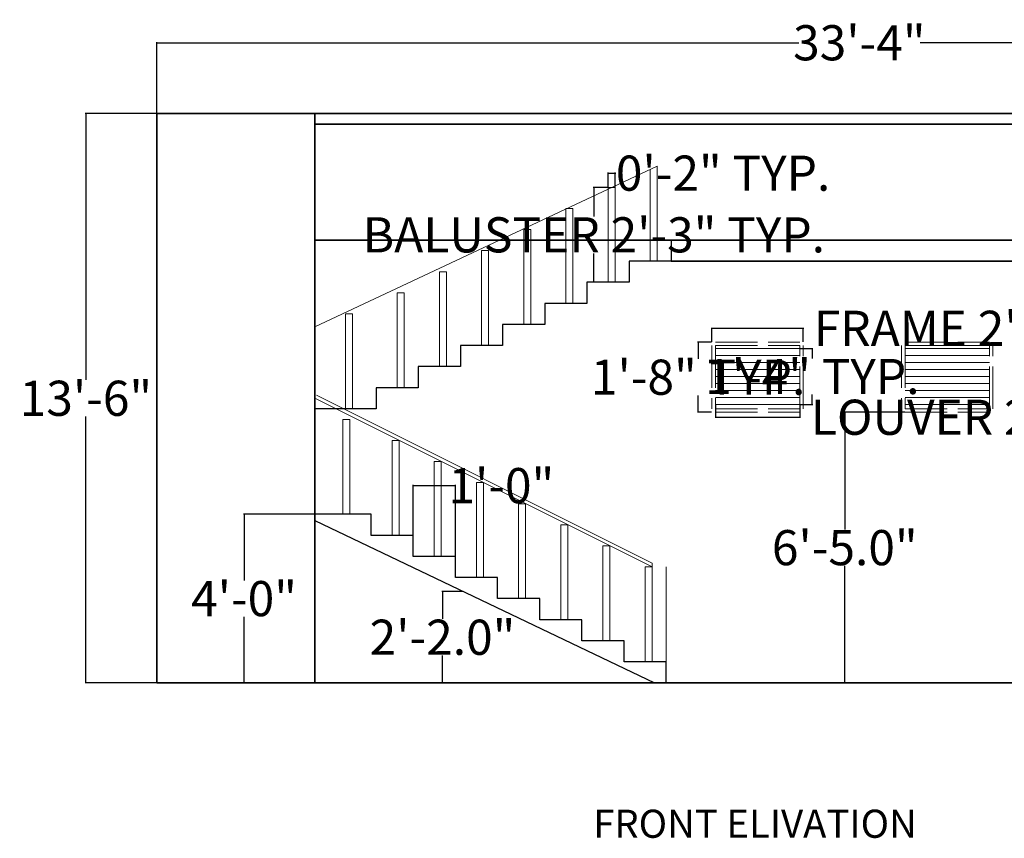
# Model space of a CAD drawing. Units: inches. Extents: x -413 to 212, y 1694 to 2633.
# Tile 1 of 5: x -378 to -98, y 1694 to 1927. Entities that reach past the tile are written whole.
import ezdxf

# ---------------------------------------------------------------- set-up
doc = ezdxf.new("R2010")
doc.units = ezdxf.units.IN
doc.header["$MEASUREMENT"] = 0
doc.linetypes.add('ACAD_ISO02W100', pattern=[15, 12, -3])
for name, color, linetype, lineweight in [('A-ANNO-DIMS', 5, 'Continuous', 18), ('A-ANNO-TEXT', 251, 'Continuous', 35), ('A-ELEV', 20, 'Continuous', 35), ('A-ELEV-RAIL', 3, 'Continuous', 18), ('A-ELEV-STRS', 3, 'Continuous', 25), ('A-ELEV-VENT', 2, 'Continuous', 18), ('A-ELEV-VENT-HIDN', 2, 'ACAD_ISO02W100', 18)]:
    doc.layers.add(name, color=color, linetype=linetype, lineweight=lineweight)
doc.styles.get("Standard").update_dxf_attribs({"font": 'arial.ttf'})
doc.dimstyles.get("Standard").update_dxf_attribs({"dimtxt": 10, "dimasz": 0.18, "dimexe": 0.18, "dimexo": 0.0625, "dimgap": 0.09, "dimtad": 0, "dimtih": 1, "dimtoh": 1, "dimdec": 1, "dimzin": 0, "dimdsep": 46, "dimlunit": 3, "dimtxsty": 'Standard', "dimblk": 'ARCHTICK', "dimcen": 0.09, "dimadec": 0, "dimazin": 0, "dimtfac": 1, "dimtdec": 1, "dimtofl": 0, "dimtmove": 0, "dimatfit": 3, "dimfxl": 1, "dimtolj": 1, "dimtzin": 0, "dimarcsym": 0})

# ---------------------------------------------------------------- blocks, each defined once
blk = doc.blocks.new('_ArchTick')
at = {"color": 0, "linetype": 'ByBlock', "const_width": 0.15}
blk.add_lwpolyline([(-0.5, -0.5), (0.5, 0.5)], dxfattribs=at)
blk = doc.blocks.new('*D9')
at = {"layer": 'A-ANNO-DIMS', "color": 0, "lineweight": -2, "transparency": 16777216}
for p, q in [((-126.04, 1815.59), (-143.33, 1815.59)), ((-143.15, 1815.59), (-143.15, 1782.28)), ((-143.15, 1738.59), (-143.15, 1771.89)), ((-126.04, 1738.59), (-143.33, 1738.59))]:
    blk.add_line(p, q, dxfattribs=at)
at = {"layer": 'Defpoints', "color": 0, "transparency": 16777216}
for p in [(-125.98, 1815.59), (-143.15, 1738.59), (-125.98, 1738.59)]:
    blk.add_point(p, dxfattribs=at)
at = {"layer": 'A-ANNO-DIMS', "color": 0, "lineweight": -2, "transparency": 16777216, "xscale": 0.18, "yscale": 0.18, "zscale": 0.18}
for p, rotation in [((-143.15, 1815.59), 90), ((-143.15, 1738.59), 270)]:
    blk.add_blockref('_ArchTick', p, dxfattribs=dict(at, rotation=rotation))
at = {"layer": 'A-ANNO-DIMS', "color": 0, "transparency": 16777216, "insert": (-143.15, 1777.09), "char_height": 10, "attachment_point": 5}
blk.add_mtext('\\A1;6\'-5.0"', dxfattribs=at)
blk = doc.blocks.new('*D10')
at = {"layer": 'A-ANNO-DIMS', "color": 0, "lineweight": -2, "transparency": 16777216}
for p, q in [((-251.8, 1764.61), (-257.82, 1764.61)), ((-257.64, 1764.61), (-257.64, 1756.79)), ((-257.64, 1738.59), (-257.64, 1746.4)), ((-252.43, 1738.59), (-257.82, 1738.59))]:
    blk.add_line(p, q, dxfattribs=at)
at = {"layer": 'Defpoints', "color": 0, "transparency": 16777216}
for p in [(-257.64, 1764.61), (-251.74, 1764.61), (-252.36, 1738.59)]:
    blk.add_point(p, dxfattribs=at)
at = {"layer": 'A-ANNO-DIMS', "color": 0, "lineweight": -2, "transparency": 16777216, "xscale": 0.18, "yscale": 0.18, "zscale": 0.18}
for p, rotation in [((-257.64, 1764.61), 90), ((-257.64, 1738.59), 270)]:
    blk.add_blockref('_ArchTick', p, dxfattribs=dict(at, rotation=rotation))
at = {"layer": 'A-ANNO-DIMS', "color": 0, "transparency": 16777216, "insert": (-257.64, 1751.6), "char_height": 10, "attachment_point": 5}
blk.add_mtext('\\A1;2\'-2.0"', dxfattribs=at)
blk = doc.blocks.new('VENT-FRAME-24X18-ELEV')
for p, q in [((1, 20), (25, 20)), ((0, 19), (0, 1)), ((1, 19), (25, 19)), ((1, 19), (1, 1)), ((25, 1), (25, 19)), ((26, 1), (26, 19)), ((1, 1), (25, 1)), ((1, 0), (25, 0))]:
    blk.add_line(p, q)
blk = doc.blocks.new('LOUVER-BLADES-24X18-ELEV')
for p, q in [((0, 16), (24, 16)), ((0, 14), (24, 14)), ((0, 12), (24, 12)), ((0, 10), (24, 10)), ((0, 8), (24, 8)), ((0, 6), (24, 6)), ((0, 4), (24, 4)), ((0, 2), (24, 2)), ((0, 0), (24, 0))]:
    blk.add_line(p, q)
blk = doc.blocks.new('BALUSTER-27IN-ELEV')
for p, q in [((0, 0), (0, 27)), ((0, 27), (2, 27)), ((2, 0), (2, 27))]:
    blk.add_line(p, q)
blk = doc.blocks.new('*D51')
at = {"layer": 'A-ANNO-DIMS', "color": 0, "lineweight": -2, "transparency": 16777216}
for p, q in [((-210.59, 1879.59), (-214.75, 1879.59)), ((-214.57, 1879.59), (-214.57, 1871.35)), ((-214.57, 1852.59), (-214.57, 1860.82)), ((-210.59, 1852.59), (-214.75, 1852.59))]:
    blk.add_line(p, q, dxfattribs=at)
at = {"layer": 'Defpoints', "color": 0, "transparency": 16777216}
for p in [(-214.57, 1879.59), (-210.52, 1879.59), (-210.52, 1852.59)]:
    blk.add_point(p, dxfattribs=at)
at = {"layer": 'A-ANNO-DIMS', "color": 0, "lineweight": -2, "transparency": 16777216, "xscale": 0.18, "yscale": 0.18, "zscale": 0.18}
for p, rotation in [((-214.57, 1879.59), 90), ((-214.57, 1852.59), 270)]:
    blk.add_blockref('_ArchTick', p, dxfattribs=dict(at, rotation=rotation))
at = {"layer": 'A-ANNO-DIMS', "color": 0, "transparency": 16777216, "insert": (-214.57, 1866.09), "char_height": 10, "attachment_point": 5}
blk.add_mtext('\\A1;BALUSTER 2\'-3" TYP.', dxfattribs=at)
blk = doc.blocks.new('*D52')
at = {"layer": 'A-ANNO-DIMS', "color": 0, "lineweight": -2, "transparency": 16777216}
for p, q in [((-210.52, 1879.65), (-210.52, 1883.82)), ((-210.52, 1883.64), (-208.52, 1883.64)), ((-208.52, 1879.65), (-208.52, 1883.82)), ((-208.52, 1883.64), (-208.34, 1883.64))]:
    blk.add_line(p, q, dxfattribs=at)
at = {"layer": 'Defpoints', "color": 0, "transparency": 16777216}
for p in [(-208.52, 1883.64), (-210.52, 1879.59), (-208.52, 1879.59)]:
    blk.add_point(p, dxfattribs=at)
at = {"layer": 'A-ANNO-DIMS', "color": 0, "lineweight": -2, "transparency": 16777216, "xscale": 0.18, "yscale": 0.18, "zscale": 0.18, "rotation": 180}
blk.add_blockref('_ArchTick', (-210.52, 1883.64), dxfattribs=at)
at = {"layer": 'A-ANNO-DIMS', "color": 0, "lineweight": -2, "transparency": 16777216, "xscale": 0.18, "yscale": 0.18, "zscale": 0.18}
blk.add_blockref('_ArchTick', (-208.52, 1883.64), dxfattribs=at)
at = {"layer": 'A-ANNO-DIMS', "color": 0, "transparency": 16777216, "insert": (-177.78, 1883.64), "char_height": 10, "attachment_point": 5}
blk.add_mtext('\\A1;0\'-2" TYP.', dxfattribs=at)
blk = doc.blocks.new('*D53')
at = {"layer": 'A-ANNO-DIMS', "color": 0, "lineweight": -2, "transparency": 16777216}
for p, q in [((-180.98, 1835.65), (-180.98, 1839.67)), ((-180.98, 1839.49), (-154.98, 1839.49)), ((-154.98, 1835.65), (-154.98, 1839.67)), ((-154.98, 1839.49), (-154.8, 1839.49))]:
    blk.add_line(p, q, dxfattribs=at)
at = {"layer": 'Defpoints', "color": 0, "transparency": 16777216}
for p in [(-154.98, 1839.49), (-180.98, 1835.59), (-154.98, 1835.59)]:
    blk.add_point(p, dxfattribs=at)
at = {"layer": 'A-ANNO-DIMS', "color": 0, "lineweight": -2, "transparency": 16777216, "xscale": 0.18, "yscale": 0.18, "zscale": 0.18, "rotation": 180}
blk.add_blockref('_ArchTick', (-180.98, 1839.49), dxfattribs=at)
at = {"layer": 'A-ANNO-DIMS', "color": 0, "lineweight": -2, "transparency": 16777216, "xscale": 0.18, "yscale": 0.18, "zscale": 0.18}
blk.add_blockref('_ArchTick', (-154.98, 1839.49), dxfattribs=at)
at = {"layer": 'A-ANNO-DIMS', "color": 0, "transparency": 16777216, "insert": (-98.12, 1839.49), "char_height": 10, "attachment_point": 5}
blk.add_mtext('\\A1;FRAME 2\'-2" TYP.', dxfattribs=at)
blk = doc.blocks.new('*D54')
at = {"layer": 'A-ANNO-DIMS', "color": 0, "lineweight": -2, "transparency": 16777216}
for p, q in [((-181.04, 1835.59), (-185.06, 1835.59)), ((-184.88, 1835.59), (-184.88, 1830.78)), ((-184.88, 1815.59), (-184.88, 1820.39)), ((-181.04, 1815.59), (-185.06, 1815.59))]:
    blk.add_line(p, q, dxfattribs=at)
at = {"layer": 'Defpoints', "color": 0, "transparency": 16777216}
for p in [(-184.88, 1835.59), (-180.98, 1835.59), (-180.98, 1815.59)]:
    blk.add_point(p, dxfattribs=at)
at = {"layer": 'A-ANNO-DIMS', "color": 0, "lineweight": -2, "transparency": 16777216, "xscale": 0.18, "yscale": 0.18, "zscale": 0.18}
for p, rotation in [((-184.88, 1835.59), 90), ((-184.88, 1815.59), 270)]:
    blk.add_blockref('_ArchTick', p, dxfattribs=dict(at, rotation=rotation))
at = {"layer": 'A-ANNO-DIMS', "color": 0, "transparency": 16777216, "insert": (-184.88, 1825.59), "char_height": 10, "attachment_point": 5}
blk.add_mtext('\\A1;1\'-8" TYP.', dxfattribs=at)
blk = doc.blocks.new('*D55')
at = {"layer": 'A-ANNO-DIMS', "color": 0, "lineweight": -2, "transparency": 16777216}
for p, q in [((-179.98, 1817.73), (-179.98, 1814.01)), ((-155.98, 1817.73), (-155.98, 1814.01)), ((-179.98, 1814.19), (-155.98, 1814.19)), ((-155.98, 1814.19), (-155.8, 1814.19))]:
    blk.add_line(p, q, dxfattribs=at)
at = {"layer": 'Defpoints', "color": 0, "transparency": 16777216}
for p in [(-179.98, 1817.79), (-155.98, 1817.79), (-155.98, 1814.19)]:
    blk.add_point(p, dxfattribs=at)
at = {"layer": 'A-ANNO-DIMS', "color": 0, "lineweight": -2, "transparency": 16777216, "xscale": 0.18, "yscale": 0.18, "zscale": 0.18, "rotation": 180}
blk.add_blockref('_ArchTick', (-179.98, 1814.19), dxfattribs=at)
at = {"layer": 'A-ANNO-DIMS', "color": 0, "lineweight": -2, "transparency": 16777216, "xscale": 0.18, "yscale": 0.18, "zscale": 0.18}
blk.add_blockref('_ArchTick', (-155.98, 1814.19), dxfattribs=at)
at = {"layer": 'A-ANNO-DIMS', "color": 0, "transparency": 16777216, "insert": (-94.78, 1814.19), "char_height": 10, "attachment_point": 5}
blk.add_mtext('\\A1;LOUVER 2\'-0" TYP.', dxfattribs=at)
blk = doc.blocks.new('*D56')
at = {"layer": 'A-ANNO-DIMS', "color": 0, "lineweight": -2, "transparency": 16777216}
for p, q in [((-155.91, 1833.79), (-152.2, 1833.79)), ((-152.38, 1833.79), (-152.38, 1830.9)), ((-152.38, 1817.79), (-152.38, 1820.68)), ((-155.91, 1817.79), (-152.2, 1817.79))]:
    blk.add_line(p, q, dxfattribs=at)
at = {"layer": 'Defpoints', "color": 0, "transparency": 16777216}
for p in [(-155.98, 1833.79), (-152.38, 1833.79), (-155.98, 1817.79)]:
    blk.add_point(p, dxfattribs=at)
at = {"layer": 'A-ANNO-DIMS', "color": 0, "lineweight": -2, "transparency": 16777216, "xscale": 0.18, "yscale": 0.18, "zscale": 0.18}
for p, rotation in [((-152.38, 1833.79), 90), ((-152.38, 1817.79), 270)]:
    blk.add_blockref('_ArchTick', p, dxfattribs=dict(at, rotation=rotation))
at = {"layer": 'A-ANNO-DIMS', "color": 0, "transparency": 16777216, "insert": (-152.38, 1825.79), "char_height": 10, "attachment_point": 5}
blk.add_mtext('\\A1;1\'-4" TYP.', dxfattribs=at)
blk = doc.blocks.new('*D60')
at = {"layer": 'A-ANNO-DIMS', "color": 0, "lineweight": -2, "transparency": 16777216}
for p, q in [((-338.98, 1900.65), (-338.98, 1920.92)), ((-338.98, 1920.74), (-156.26, 1920.74)), ((60.99, 1920.74), (-121.73, 1920.74)), ((60.99, 1900.65), (60.99, 1920.92))]:
    blk.add_line(p, q, dxfattribs=at)
at = {"layer": 'Defpoints', "color": 0, "transparency": 16777216}
for p in [(60.99, 1920.74), (-338.98, 1900.59), (60.99, 1900.59)]:
    blk.add_point(p, dxfattribs=at)
at = {"layer": 'A-ANNO-DIMS', "color": 0, "lineweight": -2, "transparency": 16777216, "xscale": 0.18, "yscale": 0.18, "zscale": 0.18, "rotation": 180}
blk.add_blockref('_ArchTick', (-338.98, 1920.74), dxfattribs=at)
at = {"layer": 'A-ANNO-DIMS', "color": 0, "lineweight": -2, "transparency": 16777216, "xscale": 0.18, "yscale": 0.18, "zscale": 0.18}
blk.add_blockref('_ArchTick', (60.99, 1920.74), dxfattribs=at)
at = {"layer": 'A-ANNO-DIMS', "color": 0, "transparency": 16777216, "insert": (-139, 1920.74), "char_height": 10, "attachment_point": 5}
blk.add_mtext('\\A1;33\'-4"', dxfattribs=at)
blk = doc.blocks.new('*D61')
at = {"layer": 'A-ANNO-DIMS', "color": 0, "lineweight": -2, "transparency": 16777216}
for p, q in [((-339.04, 1900.59), (-359.31, 1900.59)), ((-359.13, 1900.59), (-359.13, 1824.79)), ((-359.13, 1738.59), (-359.13, 1814.39)), ((-339.04, 1738.59), (-359.31, 1738.59))]:
    blk.add_line(p, q, dxfattribs=at)
at = {"layer": 'Defpoints', "color": 0, "transparency": 16777216}
for p in [(-359.13, 1900.59), (-338.98, 1900.59), (-338.98, 1738.59)]:
    blk.add_point(p, dxfattribs=at)
at = {"layer": 'A-ANNO-DIMS', "color": 0, "lineweight": -2, "transparency": 16777216, "xscale": 0.18, "yscale": 0.18, "zscale": 0.18}
for p, rotation in [((-359.13, 1900.59), 90), ((-359.13, 1738.59), 270)]:
    blk.add_blockref('_ArchTick', p, dxfattribs=dict(at, rotation=rotation))
at = {"layer": 'A-ANNO-DIMS', "color": 0, "transparency": 16777216, "insert": (-359.13, 1819.59), "char_height": 10, "attachment_point": 5}
blk.add_mtext('\\A1;13\'-6"', dxfattribs=at)
blk = doc.blocks.new('*D63')
at = {"layer": 'A-ANNO-DIMS', "color": 0, "lineweight": -2, "transparency": 16777216}
for p, q in [((-294.04, 1786.59), (-314.31, 1786.59)), ((-314.13, 1786.59), (-314.13, 1767.78)), ((-314.13, 1738.59), (-314.13, 1757.39)), ((-294.04, 1738.59), (-314.31, 1738.59))]:
    blk.add_line(p, q, dxfattribs=at)
at = {"layer": 'Defpoints', "color": 0, "transparency": 16777216}
for p in [(-314.13, 1786.59), (-293.98, 1786.59), (-293.98, 1738.59)]:
    blk.add_point(p, dxfattribs=at)
at = {"layer": 'A-ANNO-DIMS', "color": 0, "lineweight": -2, "transparency": 16777216, "xscale": 0.18, "yscale": 0.18, "zscale": 0.18}
for p, rotation in [((-314.13, 1786.59), 90), ((-314.13, 1738.59), 270)]:
    blk.add_blockref('_ArchTick', p, dxfattribs=dict(at, rotation=rotation))
at = {"layer": 'A-ANNO-DIMS', "color": 0, "transparency": 16777216, "insert": (-314.13, 1762.59), "char_height": 10, "attachment_point": 5}
blk.add_mtext('\\A1;4\'-0"', dxfattribs=at)
blk = doc.blocks.new('*D81')
at = {"layer": 'A-ANNO-DIMS', "color": 0, "lineweight": -2, "transparency": 16777216}
for p, q in [((-265.98, 1774.65), (-265.98, 1794.92)), ((-265.98, 1794.74), (-253.98, 1794.74)), ((-253.98, 1774.65), (-253.98, 1794.92)), ((-253.98, 1794.74), (-253.8, 1794.74))]:
    blk.add_line(p, q, dxfattribs=at)
at = {"layer": 'Defpoints', "color": 0, "transparency": 16777216}
for p in [(-253.98, 1794.74), (-265.98, 1774.59), (-253.98, 1774.59)]:
    blk.add_point(p, dxfattribs=at)
at = {"layer": 'A-ANNO-DIMS', "color": 0, "lineweight": -2, "transparency": 16777216, "xscale": 0.18, "yscale": 0.18, "zscale": 0.18, "rotation": 180}
blk.add_blockref('_ArchTick', (-265.98, 1794.74), dxfattribs=at)
at = {"layer": 'A-ANNO-DIMS', "color": 0, "lineweight": -2, "transparency": 16777216, "xscale": 0.18, "yscale": 0.18, "zscale": 0.18}
blk.add_blockref('_ArchTick', (-253.98, 1794.74), dxfattribs=at)
at = {"layer": 'A-ANNO-DIMS', "color": 0, "transparency": 16777216, "insert": (-240.89, 1794.74), "char_height": 10, "attachment_point": 5}
blk.add_mtext('\\A1;1\'-0"', dxfattribs=at)

msp = doc.modelspace()

# ---------------------------------------------------------------- linework, layer by layer
at = {"layer": 'A-ELEV'}
for p, q in [((-338.98, 1900.59), (60.99, 1900.59)), ((-338.98, 1900.59), (-338.98, 1738.59)), ((-293.98, 1900.59), (-293.98, 1738.59)), ((-293.98, 1897.59), (60.99, 1897.59)), ((-293.98, 1864.59), (60.99, 1864.59)), ((-192.52, 1858.59), (60.99, 1858.59)), ((-338.98, 1738.59), (60.99, 1738.59))]:
    msp.add_line(p, q, dxfattribs=at)
at = {"layer": 'A-ELEV-RAIL'}
for p, q in [((-196.52, 1885.59), (-293.98, 1839.92)), ((-198.52, 1858.59), (-198.52, 1884.65)), ((-196.52, 1858.59), (-196.52, 1885.59)), ((-197.98, 1771.59), (-293.98, 1819.59)), ((-197.98, 1772.71), (-293.53, 1820.48)), ((-199.98, 1744.59), (-199.98, 1771.59)), ((-199.98, 1771.59), (-197.98, 1771.59)), ((-197.98, 1744.59), (-197.98, 1772.71)), ((-193.98, 1744.59), (-193.98, 1771.59)), ((-193.98, 1771.59), (-193.98, 1738.59))]:
    msp.add_line(p, q, dxfattribs=at)
at = {"layer": 'A-ELEV-STRS'}
for p, q in [((-192.52, 1864.59), (-192.52, 1858.59)), ((-192.52, 1858.59), (-204.52, 1858.59)), ((-204.52, 1858.59), (-204.52, 1852.59)), ((-204.52, 1852.59), (-216.52, 1852.59)), ((-216.52, 1852.59), (-216.52, 1846.59)), ((-216.52, 1846.59), (-228.52, 1846.59)), ((-228.52, 1846.59), (-228.52, 1840.59)), ((-228.52, 1840.59), (-240.52, 1840.59)), ((-240.52, 1840.59), (-240.52, 1834.59)), ((-240.52, 1834.59), (-252.52, 1834.59)), ((-252.52, 1834.59), (-252.52, 1828.59)), ((-252.52, 1828.59), (-264.52, 1828.59)), ((-264.52, 1828.59), (-264.52, 1822.59)), ((-264.52, 1822.59), (-276.52, 1822.59)), ((-276.52, 1822.59), (-276.52, 1816.59)), ((-276.52, 1816.59), (-293.98, 1816.59)), ((-293.98, 1786.59), (-293.98, 1792.59)), ((-277.98, 1786.59), (-293.98, 1786.59)), ((-277.98, 1780.59), (-277.98, 1786.59)), ((-293.98, 1784.81), (-197.34, 1738.59)), ((-265.98, 1780.59), (-277.98, 1780.59)), ((-265.98, 1774.59), (-265.98, 1780.59)), ((-253.98, 1774.59), (-265.98, 1774.59)), ((-253.98, 1768.59), (-253.98, 1774.59)), ((-241.98, 1768.59), (-253.98, 1768.59)), ((-241.98, 1762.59), (-241.98, 1768.59)), ((-229.98, 1762.59), (-241.98, 1762.59)), ((-229.98, 1756.59), (-229.98, 1762.59)), ((-217.98, 1756.59), (-229.98, 1756.59)), ((-217.98, 1750.59), (-217.98, 1756.59)), ((-205.98, 1750.59), (-217.98, 1750.59)), ((-205.98, 1744.59), (-205.98, 1750.59)), ((-193.98, 1744.59), (-205.98, 1744.59)), ((-193.98, 1738.59), (-193.98, 1744.59))]:
    msp.add_line(p, q, dxfattribs=at)
at = {"layer": 'A-ELEV-VENT'}
msp.add_line((-155.98, 1833.79), (-154.98, 1833.79), dxfattribs=at)

# ---------------------------------------------------------------- block references
at = {"layer": 'A-ELEV-RAIL'}
for p in [(-210.52, 1852.59), (-222.52, 1846.59), (-234.52, 1840.59), (-246.52, 1834.59), (-258.52, 1828.59), (-270.52, 1822.59), (-285.25, 1816.59), (-285.98, 1786.59), (-271.98, 1780.59), (-259.98, 1774.59), (-247.98, 1768.59), (-235.98, 1762.59), (-223.98, 1756.59), (-211.98, 1750.59)]:
    msp.add_blockref('BALUSTER-27IN-ELEV', p, dxfattribs=at)
at = {"layer": 'A-ELEV-VENT'}
msp.add_blockref('LOUVER-BLADES-24X18-ELEV', (-179.98, 1817.79), dxfattribs=at)
at = {"layer": 'A-ELEV-VENT', "rotation": 180}
msp.add_blockref('LOUVER-BLADES-24X18-ELEV', (-101.98, 1833.79), dxfattribs=at)
at = {"layer": 'A-ELEV-VENT-HIDN'}
for p in [(-180.98, 1815.59), (-126.98, 1815.59)]:
    msp.add_blockref('VENT-FRAME-24X18-ELEV', p, dxfattribs=at)

# ---------------------------------------------------------------- texts
at = {"layer": 'A-ANNO-TEXT'}
msp.add_text('FRONT ELIVATION', height=8, dxfattribs=at).set_placement((-214.76, 1694.53))

# ---------------------------------------------------------------- dimensions: what is measured, and where the dimension line sits
at = {"layer": 'A-ANNO-DIMS'}
for base, p1, p2, picture, middle in [((60.99, 1920.74), (-338.98, 1900.59), (60.99, 1900.59), '*D60', (-139, 1920.74)), ((-253.98, 1794.74), (-265.98, 1774.59), (-253.98, 1774.59), '*D81', (-240.89, 1794.74))]:
    dim = msp.add_linear_dim(base=base, p1=p1, p2=p2, dimstyle='Standard', override={"dimdec": 1, "dimlfac": 1, "dimrnd": 0, "dimzin": 1, "dimdsep": 46, "dimlunit": 4, "dimfrac": 2}, dxfattribs=at)
    dim.commit()
    dim.dimension.update_dxf_attribs({"geometry": picture, "text_midpoint": middle})
for base, p1, p2, override, picture, middle in [((-359.13, 1900.59), (-338.98, 1738.59), (-338.98, 1900.59), {"dimdec": 1, "dimlfac": 1, "dimrnd": 0, "dimzin": 1, "dimdsep": 46, "dimlunit": 4, "dimfrac": 2}, '*D61', (-359.13, 1819.59)), ((-143.15, 1738.59), (-125.98, 1815.59), (-125.98, 1738.59), {"dimclrd": 0, "dimclre": 0, "dimclrt": 0}, '*D9', (-143.15, 1777.09)), ((-314.13, 1786.59), (-293.98, 1738.59), (-293.98, 1786.59), {"dimdec": 1, "dimlfac": 1, "dimrnd": 0, "dimzin": 1, "dimdsep": 46, "dimlunit": 4, "dimfrac": 2}, '*D63', (-314.13, 1762.59)), ((-257.64, 1764.61), (-252.36, 1738.59), (-251.74, 1764.61), {"dimclrd": 0, "dimclre": 0, "dimclrt": 0}, '*D10', (-257.64, 1751.6))]:
    dim = msp.add_linear_dim(base=base, p1=p1, p2=p2, angle=90, dimstyle='Standard', override=override, dxfattribs=at)
    dim.commit()
    dim.dimension.update_dxf_attribs({"geometry": picture, "text_midpoint": middle})
for base, p1, p2, text, picture, middle in [((-208.52, 1883.64), (-210.52, 1879.59), (-208.52, 1879.59), '<> TYP.', '*D52', (-177.78, 1883.64)), ((-154.98, 1839.49), (-180.98, 1835.59), (-154.98, 1835.59), 'FRAME <> TYP.', '*D53', (-98.12, 1839.49)), ((-155.98, 1814.19), (-179.98, 1817.79), (-155.98, 1817.79), 'LOUVER <> TYP.', '*D55', (-94.78, 1814.19))]:
    dim = msp.add_linear_dim(base=base, p1=p1, p2=p2, text=text, dimstyle='Standard', override={"dimdec": 1, "dimlfac": 1, "dimrnd": 0, "dimzin": 1, "dimdsep": 46, "dimlunit": 4, "dimfrac": 2}, dxfattribs=at)
    dim.commit()
    dim.dimension.update_dxf_attribs({"geometry": picture, "text_midpoint": middle})
for base, p1, p2, text, picture, middle in [((-214.57, 1879.59), (-210.52, 1852.59), (-210.52, 1879.59), 'BALUSTER <> TYP.', '*D51', (-214.57, 1866.09)), ((-184.88, 1835.59), (-180.98, 1815.59), (-180.98, 1835.59), '<> TYP.', '*D54', (-184.88, 1825.59)), ((-152.38, 1833.79), (-155.98, 1817.79), (-155.98, 1833.79), '<> TYP.', '*D56', (-152.38, 1825.79))]:
    dim = msp.add_linear_dim(base=base, p1=p1, p2=p2, angle=90, text=text, dimstyle='Standard', override={"dimdec": 1, "dimlfac": 1, "dimrnd": 0, "dimzin": 1, "dimdsep": 46, "dimlunit": 4, "dimfrac": 2}, dxfattribs=at)
    dim.commit()
    dim.dimension.update_dxf_attribs({"geometry": picture, "text_midpoint": middle})

doc.saveas('drawing.dxf')
